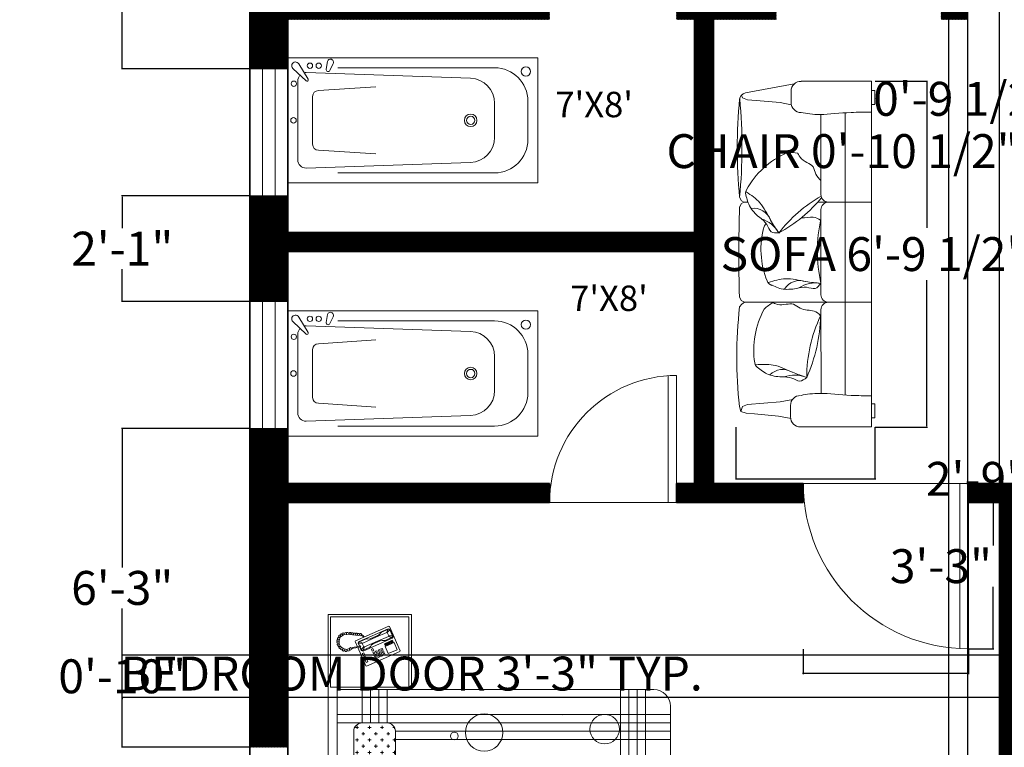
# Model space of a CAD drawing. Units: inches. Extents: x 108 to 771, y 58 to 590.
# Tile 2 of 8: x 108 to 341, y 231 to 402. Entities that reach past the tile are written whole.
import ezdxf

# ---------------------------------------------------------------- set-up
doc = ezdxf.new("R2010")
doc.units = ezdxf.units.IN
doc.header["$MEASUREMENT"] = 0
for name, color, linetype, lineweight in [('A-ANNO-DIMS', 2, 'Continuous', 13), ('A-AREA-IDEN', 7, 'Continuous', 18), ('A-DOOR', 3, 'Continuous', 18), ('A-FLOR-FIXT', 8, 'Continuous', 15), ('A-GLAZ', 4, 'Continuous', 18), ('A-WALL', 7, 'Continuous', 35), ('A-WALL-PATT', 252, 'Continuous', 9), ('Furniture', 7, 'Continuous', 15)]:
    doc.layers.add(name, color=color, linetype=linetype, lineweight=lineweight)
doc.styles.get("Standard").update_dxf_attribs({"font": 'italic8.shx'})
doc.dimstyles.get("Standard").update_dxf_attribs({"dimtxt": 8, "dimasz": 0.18, "dimexe": 0.18, "dimexo": 0.0625, "dimgap": 0.09, "dimtad": 0, "dimtih": 1, "dimtoh": 1, "dimzin": 0, "dimdsep": 46, "dimlunit": 3, "dimtxsty": 'Standard', "dimcen": 0.09, "dimclrt": 6, "dimadec": 0, "dimazin": 0, "dimtfac": 1, "dimtofl": 0, "dimtmove": 0, "dimatfit": 3, "dimfxl": 1, "dimtolj": 1, "dimtzin": 0, "dimarcsym": 0})

# ---------------------------------------------------------------- blocks, each defined once
blk = doc.blocks.new('DOOR-SINGLE-39')
for p, q in [((0, 39), (0, 0)), ((2, 38.95), (2, 0)), ((0, 0), (39, 0))]:
    blk.add_line(p, q)
blk.add_arc((0, 0), 39, 0, 90)
blk = doc.blocks.new('DOOR-SINGLE-30')
for p, q in [((28, 29.93), (28, 0)), ((30, 30), (30, 0)), ((30, 0), (0, 0))]:
    blk.add_line(p, q)
blk.add_arc((30, 0), 30, 90, 180)
blk = doc.blocks.new('WINDOW-30')
for p, q in [((0, 0), (0, 30)), ((0, 30), (9, 30)), ((3, 30), (3, 0)), ((6, 30), (6, 0)), ((9, 30), (9, 0)), ((9, 0), (0, 0))]:
    blk.add_line(p, q)
blk = doc.blocks.new('BED-WITH-NIGHTSTANDS')
h = blk.add_hatch()
h.set_pattern_fill('CROSS', color=256, scale=5.9055, angle=450, style=0)
h.set_pattern_definition([(90, (-724.7189, -618.2251), (1.476375, 1.476375), [0.7381875, -2.2145625]), (360, (-725.088, -617.856), (1.476375, -1.476375), [0.7381875, -2.2145625])])
h.paths.add_polyline_path([(13.93, 48.57), (8.02, 48.57, 0.414214), (6.06, 46.6), (6.06, 28.74, 0.414214), (8.02, 26.77), (13.93, 26.77, 0.414214), (15.9, 28.74), (15.9, 46.6, 0.414214)])
h.paths.add_polyline_path([(6.06, 62.99, 0.19223), (8.02, 57.33), (13.93, 57.33, 0.19223), (15.9, 62.99), (15.9, 78.74, 0.414214), (13.93, 80.71), (8.02, 80.71, 0.414214), (6.06, 78.74)])
for p, q in [((0, 0), (0, 106.3)), ((19.69, 106.3), (0, 106.3)), ((19.09, 105.71), (0.59, 105.71)), ((0.59, 105.71), (0.59, 89.17)), ((19.09, 105.71), (19.09, 89.17)), ((19.69, 106.3), (19.69, 88.58)), ((14.35, 103.55), (6.45, 100.09)), ((14.21, 102.94), (7.34, 99.94)), ((14.14, 102.78), (12.6, 102.1)), ((14.14, 102.78), (13.85, 102.03)), ((13.99, 102.03), (14.61, 102.64)), ((14.4, 102.82), (14.14, 102.78)), ((14.62, 102.78), (14.21, 102.94)), ((14.52, 103.48), (14.35, 103.55)), ((14.61, 102.64), (14.4, 102.82)), ((17.02, 97.76), (14.52, 103.48)), ((15.21, 101.26), (14.61, 102.64)), ((15.37, 101.06), (14.62, 102.78)), ((2.06, 100.15), (2.14, 100.41)), ((2.46, 100.04), (2.06, 100.15)), ((2.1, 99.92), (2.46, 100.04)), ((2.14, 100.41), (2.51, 100.41)), ((2.23, 100.67), (2.3, 100.88)), ((2.51, 100.41), (2.23, 100.67)), ((2.3, 100.88), (2.69, 100.86)), ((2.44, 101.15), (2.63, 101.34)), ((2.69, 100.86), (2.44, 101.15)), ((2.89, 100.92), (2.62, 100.19)), ((2.62, 100.19), (2.62, 99.39)), ((2.63, 101.34), (3.06, 101.2)), ((2.89, 101.55), (3.11, 101.7)), ((3.06, 101.2), (2.89, 101.55)), ((3.69, 101.46), (2.89, 100.92)), ((3.11, 101.7), (3.41, 101.48)), ((3.36, 101.88), (3.67, 101.95)), ((3.41, 101.48), (3.36, 101.88)), ((3.67, 101.95), (3.81, 101.64)), ((4.95, 101.56), (3.69, 101.46)), ((3.81, 101.64), (3.94, 101.98)), ((3.94, 101.98), (4.24, 102.02)), ((4.24, 102.02), (4.39, 101.64)), ((4.37, 102.03), (4.76, 102.08)), ((4.39, 101.64), (4.37, 102.03)), ((4.76, 102.08), (4.88, 101.72)), ((4.88, 101.72), (5.13, 102.07)), ((5.79, 101.48), (4.95, 101.56)), ((5.13, 102.07), (5.37, 102.03)), ((5.37, 102.03), (5.42, 101.66)), ((5.42, 101.66), (5.65, 101.97)), ((5.65, 101.97), (5.95, 101.95)), ((5.86, 101.55), (5.79, 101.48)), ((5.92, 101.48), (5.86, 101.55)), ((6.5, 101.45), (5.92, 101.48)), ((5.95, 101.95), (5.98, 101.59)), ((5.98, 101.59), (6.16, 101.92)), ((6.16, 101.92), (6.47, 101.91)), ((6.45, 100.09), (6.38, 99.93)), ((6.47, 101.91), (6.46, 101.54)), ((6.46, 101.54), (6.62, 101.9)), ((7.29, 101.35), (6.5, 101.45)), ((6.62, 101.9), (6.85, 101.89)), ((6.85, 101.89), (6.89, 101.51)), ((6.89, 101.51), (7.15, 101.84)), ((7.15, 101.84), (7.36, 101.82)), ((7.73, 101.29), (7.29, 101.35)), ((7.36, 101.82), (7.4, 101.48)), ((7.4, 101.48), (7.62, 101.8)), ((7.44, 99.85), (8.99, 100.52)), ((7.62, 101.8), (7.77, 101.81)), ((7.79, 101.48), (7.73, 101.29)), ((7.77, 101.81), (7.86, 101.7)), ((7.84, 101.37), (7.79, 101.48)), ((7.94, 101.33), (7.84, 101.37)), ((7.86, 101.7), (7.96, 101.49)), ((8.11, 101.22), (7.94, 101.33)), ((7.96, 101.49), (8.25, 101.43)), ((8.26, 101.14), (8.11, 101.22)), ((11.28, 100.91), (8.18, 99.56)), ((8.25, 101.43), (8.4, 101.32)), ((8.4, 100.95), (8.26, 101.14)), ((8.26, 97.68), (15.18, 100.71)), ((8.4, 101.32), (8.57, 101.02)), ((11.68, 99.99), (8.58, 98.64)), ((8.99, 100.52), (9.33, 100.53)), ((9.33, 100.53), (9.69, 100.49)), ((9.69, 100.49), (10.11, 100.6)), ((10.11, 100.6), (11.2, 101.08)), ((11.77, 101.33), (11.2, 101.08)), ((11.28, 100.91), (13.85, 102.03)), ((11.68, 99.99), (14.25, 101.12)), ((12.33, 100.07), (11.75, 99.82)), ((12.15, 101.56), (11.77, 101.33)), ((12.36, 101.86), (12.15, 101.56)), ((12.75, 100.19), (12.33, 100.07)), ((12.6, 102.1), (12.36, 101.86)), ((13.11, 100.14), (12.75, 100.19)), ((13.45, 100.15), (13.11, 100.14)), ((15, 100.83), (13.45, 100.15)), ((13.85, 102.03), (13.99, 102.03)), ((13.99, 102.03), (14.34, 101.23)), ((14.25, 101.12), (14.34, 101.23)), ((15, 100.83), (14.25, 101.12)), ((14.34, 101.23), (15.21, 101.26)), ((14.67, 100), (14.84, 100.08)), ((14.87, 99.55), (14.67, 100)), ((14.84, 100.08), (15.04, 99.62)), ((15.2, 100.99), (15, 100.83)), ((15.02, 100.16), (15.19, 100.23)), ((15.22, 99.7), (15.02, 100.16)), ((15.18, 100.71), (15.37, 101.06)), ((15.19, 100.23), (15.39, 99.77)), ((15.21, 101.26), (15.2, 100.99)), ((2.09, 99.7), (2.1, 99.92)), ((2.44, 99.53), (2.09, 99.7)), ((2.13, 99.38), (2.44, 99.53)), ((2.17, 99.14), (2.13, 99.38)), ((2.59, 99.17), (2.17, 99.14)), ((2.29, 98.95), (2.59, 99.17)), ((2.4, 98.76), (2.29, 98.95)), ((2.78, 98.76), (2.4, 98.76)), ((2.53, 98.47), (2.78, 98.76)), ((2.71, 98.26), (2.53, 98.47)), ((2.62, 99.39), (2.98, 98.72)), ((3.07, 98.46), (2.71, 98.26)), ((2.96, 98.08), (3.07, 98.46)), ((3.2, 97.92), (2.96, 98.08)), ((2.98, 98.72), (3.58, 98.25)), ((3.49, 98.1), (3.2, 97.92)), ((3.41, 97.75), (3.49, 98.1)), ((3.69, 97.67), (3.41, 97.75)), ((3.58, 98.25), (4.33, 98.05)), ((3.95, 97.97), (3.69, 97.67)), ((4.03, 97.59), (3.95, 97.97)), ((4.33, 98.05), (5.08, 98.31)), ((4.48, 97.99), (4.36, 97.56)), ((4.67, 97.64), (4.48, 97.99)), ((5, 97.75), (4.67, 97.64)), ((5.05, 98.16), (5, 97.75)), ((5.26, 97.85), (5.05, 98.16)), ((5.08, 98.31), (5.33, 98.48)), ((5.53, 98), (5.26, 97.85)), ((5.33, 98.48), (5.57, 98.34)), ((5.6, 98.18), (5.53, 98)), ((5.57, 98.34), (5.87, 98.48)), ((5.68, 98.18), (5.6, 98.18)), ((5.98, 98.32), (5.68, 98.18)), ((5.87, 98.48), (6.16, 98.57)), ((6.58, 98.42), (5.98, 98.32)), ((6.16, 98.57), (6.77, 98.66)), ((6.38, 99.93), (6.92, 98.7)), ((7.22, 98.53), (6.58, 98.42)), ((6.77, 98.66), (7.17, 98.75)), ((7.01, 98.5), (8.89, 94.2)), ((7.34, 99.94), (7.12, 99.5)), ((7.12, 99.5), (7.41, 98.83)), ((7.17, 98.75), (7.65, 98.91)), ((7.72, 98.74), (7.22, 98.53)), ((7.23, 99.41), (7.24, 99.69)), ((8.09, 99.45), (7.23, 99.41)), ((7.47, 98.85), (7.23, 99.41)), ((7.24, 99.69), (7.44, 99.85)), ((7.44, 99.85), (8.18, 99.56)), ((7.49, 98.64), (7.84, 97.84)), ((7.83, 98.04), (7.55, 98.67)), ((7.65, 98.91), (7.72, 98.74)), ((8.45, 98.65), (7.83, 98.04)), ((7.83, 98.04), (8.04, 97.86)), ((7.84, 97.84), (8.26, 97.68)), ((8.04, 97.86), (8.29, 97.9)), ((8.18, 99.56), (8.09, 99.45)), ((8.09, 99.45), (8.45, 98.65)), ((8.29, 97.9), (8.58, 98.64)), ((8.29, 97.9), (9.84, 98.58)), ((8.58, 98.64), (8.45, 98.65)), ((9.84, 98.58), (10.08, 98.82)), ((10.08, 98.82), (10.29, 99.11)), ((10.58, 98.29), (10.24, 98.14)), ((10.24, 98.14), (10.44, 97.68)), ((10.29, 99.11), (10.66, 99.34)), ((10.44, 97.68), (10.78, 97.83)), ((10.78, 97.83), (10.58, 98.29)), ((10.66, 99.34), (11.75, 99.82)), ((11.56, 97.76), (11.22, 97.61)), ((11.71, 97.42), (11.56, 97.76)), ((12.19, 98.03), (11.85, 97.88)), ((11.85, 97.88), (12, 97.54)), ((12, 97.54), (12.34, 97.69)), ((12.34, 97.69), (12.19, 98.03)), ((12.82, 98.31), (12.48, 98.16)), ((12.48, 98.16), (12.63, 97.82)), ((12.63, 97.82), (12.97, 97.97)), ((13.07, 97.74), (12.73, 97.59)), ((12.97, 97.97), (12.82, 98.31)), ((13.22, 97.39), (13.07, 97.74)), ((13.3, 99.4), (13.47, 99.48)), ((13.5, 98.95), (13.3, 99.4)), ((15.58, 99.65), (13.46, 98.72)), ((13.46, 98.72), (14.18, 97.06)), ((13.47, 99.48), (13.67, 99.02)), ((13.67, 99.02), (13.5, 98.95)), ((13.64, 99.55), (13.81, 99.63)), ((13.84, 99.1), (13.64, 99.55)), ((13.81, 99.63), (14.01, 99.17)), ((14.01, 99.17), (13.84, 99.1)), ((13.99, 99.7), (14.16, 99.78)), ((14.19, 99.25), (13.99, 99.7)), ((14.16, 99.78), (14.36, 99.32)), ((14.18, 97.06), (16.3, 97.99)), ((14.36, 99.32), (14.19, 99.25)), ((14.33, 99.85), (14.5, 99.93)), ((14.53, 99.4), (14.33, 99.85)), ((14.5, 99.93), (14.7, 99.47)), ((14.7, 99.47), (14.53, 99.4)), ((15.04, 99.62), (14.87, 99.55)), ((15.39, 99.77), (15.22, 99.7)), ((16.3, 97.99), (15.58, 99.65)), ((16.96, 97.59), (17.02, 97.76)), ((4.36, 97.56), (4.03, 97.59)), ((8.09, 97.13), (8.43, 97.28)), ((8.34, 96.55), (8.09, 97.13)), ((8.68, 96.7), (8.34, 96.55)), ((8.43, 97.28), (8.68, 96.7)), ((8.44, 96.33), (8.78, 96.48)), ((8.69, 95.75), (8.44, 96.33)), ((9.03, 95.9), (8.69, 95.75)), ((8.78, 96.48), (9.03, 95.9)), ((8.79, 95.52), (9.13, 95.67)), ((9.04, 94.95), (8.79, 95.52)), ((9.05, 94.14), (16.96, 97.59)), ((9.13, 95.67), (9.38, 95.1)), ((10.93, 97.48), (10.59, 97.33)), ((10.59, 97.33), (10.74, 96.99)), ((10.74, 96.99), (11.08, 97.14)), ((11.18, 96.91), (10.84, 96.76)), ((10.84, 96.76), (10.99, 96.42)), ((11.08, 97.14), (10.93, 97.48)), ((10.99, 96.42), (11.33, 96.57)), ((11.43, 96.34), (11.09, 96.19)), ((11.09, 96.19), (11.24, 95.84)), ((11.33, 96.57), (11.18, 96.91)), ((11.22, 97.61), (11.37, 97.27)), ((11.24, 95.84), (11.58, 95.99)), ((11.37, 97.27), (11.71, 97.42)), ((11.58, 95.99), (11.43, 96.34)), ((11.81, 97.19), (11.47, 97.04)), ((11.47, 97.04), (11.62, 96.69)), ((11.62, 96.69), (11.96, 96.84)), ((12.06, 96.61), (11.72, 96.46)), ((11.72, 96.46), (11.87, 96.12)), ((11.96, 96.84), (11.81, 97.19)), ((11.87, 96.12), (12.21, 96.27)), ((12.21, 96.27), (12.06, 96.61)), ((12.44, 97.46), (12.1, 97.31)), ((12.1, 97.31), (12.25, 96.97)), ((12.25, 96.97), (12.59, 97.12)), ((12.69, 96.89), (12.35, 96.74)), ((12.35, 96.74), (12.5, 96.39)), ((12.59, 97.12), (12.44, 97.46)), ((12.5, 96.39), (12.84, 96.55)), ((12.84, 96.55), (12.69, 96.89)), ((12.73, 97.59), (12.88, 97.24)), ((12.88, 97.24), (13.22, 97.39)), ((13.32, 97.16), (12.98, 97.01)), ((12.98, 97.01), (13.13, 96.67)), ((13.13, 96.67), (13.47, 96.82)), ((13.47, 96.82), (13.32, 97.16)), ((8.89, 94.2), (9.05, 94.14)), ((9.38, 95.1), (9.04, 94.95)), ((19.09, 89.17), (0.59, 89.17)), ((0.59, 89.17), (19.09, 89.17)), ((2.12, 17.72), (2.12, 88.58)), ((2.12, 88.58), (76.92, 88.58)), ((80.86, 84.65), (80.86, 21.65)), ((55.34, 82.68), (55.28, 82.62)), ((6.07, 78.98), (6.07, 62.76)), ((6.07, 46.84), (6.07, 28.51)), ((6.07, 44.57), (6.06, 44.56)), ((50.36, 26.51), (46.1, 22.26)), ((19.09, 17.13), (0.59, 17.13)), ((0.59, 0.59), (0.59, 17.13)), ((76.92, 17.72), (2.12, 17.72)), ((19.09, 0.59), (19.09, 17.13)), ((19.69, 0), (19.69, 17.72)), ((9.61, 8.71), (9.61, 14.05)), ((8.07, 10.1), (5.65, 12.3)), ((11, 10.24), (13.2, 12.67)), ((9.61, 8.71), (4.26, 8.71)), ((8.22, 7.18), (6.02, 4.75)), ((9.61, 8.71), (14.95, 8.71)), ((9.61, 8.71), (9.61, 3.36)), ((11.14, 7.32), (13.56, 5.12)), ((19.69, 0), (0, 0)), ((19.09, 0.59), (0.59, 0.59))]:
    blk.add_line(p, q)
for points in [[(8.02, 88.58), (8.02, 80.71)], [(9.99, 80.71), (9.99, 88.58), (8.02, 88.58)], [(13.93, 80.71), (13.93, 88.58), (11.96, 88.58)], [(11.96, 88.58), (11.96, 80.71)], [(2.12, 80.71), (80.86, 80.71), (80.86, 82.68), (2.12, 82.68)], [(15.9, 76.77), (80.86, 76.77), (80.86, 78.74), (15.9, 78.74)], [(8.02, 57.33), (8.02, 48.57)], [(9.99, 48.57), (9.99, 57.33)], [(11.96, 57.33), (11.96, 48.57)], [(13.93, 48.57), (13.93, 57.33)], [(2.12, 29.53), (6.06, 29.53)], [(15.9, 29.53), (80.86, 29.53), (80.86, 27.56), (15.9, 27.56)], [(6.06, 27.56), (2.12, 27.56)], [(2.12, 25.59), (80.86, 25.59), (80.86, 23.62), (2.12, 23.62)], [(8.02, 25.59), (8.02, 17.72), (9.99, 17.72), (9.99, 25.59)], [(11.96, 25.59), (11.96, 17.72), (13.93, 17.72), (13.93, 25.59)]]:
    blk.add_lwpolyline(points)
for points in [[(69.05, 88.58), (69.05, 17.72), (71.02, 17.72), (71.02, 88.58)], [(72.98, 88.58), (72.98, 17.72), (74.95, 17.72), (74.95, 88.58)]]:
    blk.add_lwpolyline(points, close=True)
for points in [[(15.9, 62.99), (15.9, 78.74, 0.414214), (13.93, 80.71), (8.02, 80.71, 0.414214), (6.06, 78.74), (6.06, 62.99, 0.19223), (8.02, 57.33), (13.93, 57.33, 0.19223)], [(15.9, 28.74), (15.9, 46.6, 0.414214), (13.93, 48.57), (8.02, 48.57, 0.414214), (6.06, 46.6), (6.06, 28.74, 0.414214), (8.02, 26.77), (13.93, 26.77, 0.414214)]]:
    blk.add_lwpolyline(points, format="xyb", close=True)
for centre, radius in [((36.86, 78.44), 4.41), ((65.32, 79.25), 3.48), ((29.81, 77.62), 0.925), ((20.97, 68.13), 2.09), ((65.3, 65.16), 2.09), ((68.02, 44.43), 4.65), ((28.31, 37.66), 4.65), ((46.05, 37.48), 0.925), ((60.91, 32.6), 1.14), ((71.58, 30.51), 2.09), ((46.4, 25.43), 3.19), ((9.61, 8.71), 5.54), ((9.61, 8.71), 5.34), ((9.61, 8.71), 2.07)]:
    blk.add_circle(centre, radius)
for centre, start, end in [((76.92, 84.65), 0, 90), ((76.92, 21.65), 270, 0)]:
    blk.add_arc(centre, 3.94, start, end)
blk = doc.blocks.new('BATHTUB')
for p, q in [((59.06, 29.53), (0, 29.53)), ((0, 29.53), (0, 0)), ((4.78, 24.45), (2.59, 28.08)), ((9.35, 28.65), (9.04, 26.82)), ((9.94, 26.54), (10.7, 28.16)), ((59.06, 0), (59.06, 29.53)), ((1.15, 27.02), (4.3, 24.06)), ((4.33, 26.04), (43.12, 24.68)), ((48.82, 27.17), (11.81, 27.17)), ((2.36, 24.07), (2.36, 5.46)), ((7.23, 21.79), (20.76, 22.69)), ((5.85, 20.41), (5.85, 9.11)), ((48.82, 10.75), (48.82, 19.29)), ((56.69, 10.24), (56.69, 19.29)), ((7.23, 7.74), (20.76, 6.84)), ((4.33, 3.49), (43.12, 4.85)), ((11.81, 2.36), (48.82, 2.36)), ((0, 0), (59.06, 0))]:
    blk.add_line(p, q)
for centre, radius in [((5.23, 27.66), 0.628), ((7.29, 27.66), 0.628), ((56.21, 26.29), 1.09), ((1.42, 23.41), 0.628), ((1.34, 14.76), 0.656), ((43.18, 14.76), 1.48), ((43.18, 14.76), 0.984)]:
    blk.add_circle(centre, radius)
for centre, radius, start, end in [((1.81, 27.63), 0.903, 29.9808, 223.0225), ((10.05, 28.48), 0.722, 333.7022, 166.7439), ((4.33, 24.07), 1.97, 90, 103.842), ((4.33, 24.07), 1.97, 90, 103.842), ((9.51, 26.74), 0.472, 170.4963, 334.8002), ((48.82, 19.29), 7.87, 0, 90), ((4.33, 24.07), 1.97, 137.6863, 180), ((4.33, 24.07), 1.97, 137.6863, 180), ((4.51, 24.29), 0.315, 226.7749, 31.0788), ((4.51, 24.29), 0.315, 226.7749, 31.0788), ((42.91, 18.78), 5.91, 0, 87.9984), ((7.23, 20.41), 1.38, 90, 180), ((42.91, 10.75), 5.91, 272.0016, 0), ((48.82, 10.24), 7.87, 270, 0), ((7.23, 9.11), 1.38, 180, 270), ((4.33, 5.46), 1.97, 180, 270)]:
    blk.add_arc(centre, radius, start, end)
blk = doc.blocks.new('SOFA')
for p, q in [((31.83, 81.57, 13.5), (15.2, 81.57, 13.5)), ((31.83, 81.57, 13.5), (31.83, 0)), ((13.53, 80.95), (2.06, 78.82)), ((12.83, 79.28), (12.82, 76.57)), ((31.83, 79.37, 0.36), (32.62, 79.37, 0.36)), ((32.62, 79.37, 0.36), (32.62, 76.1, 0.36)), ((1.33, 77.65), (1.12, 78.32)), ((2.53, 77.19), (1.33, 77.65)), ((4.58, 77.03), (2.53, 77.19)), ((10.24, 76.55), (4.58, 77.03)), ((12.88, 76.04), (10.24, 76.55)), ((32.62, 76.1, 0.36), (31.83, 76.1, 0.91)), ((19.88, 73.73), (19.88, 54.83)), ((25.57, 7.53, 9.89), (25.57, 74.14, 9.89)), ((1.09, 53.34), (0.67, 54.21)), ((1.09, 52.77), (0.68, 51.91)), ((1.64, 53.06), (1.09, 53.34)), ((1.64, 53.06), (1.09, 52.77)), ((1.64, 53.06), (2.64, 53.06)), ((19.09, 53.06), (21.65, 53.06)), ((19.88, 51.29), (19.88, 31.21)), ((21.65, 53.06), (31.83, 53.06)), ((1.05, 29.87), (0.64, 30.74)), ((1.19, 29.01), (0.68, 28.32)), ((1.8, 29.44), (1.05, 29.87)), ((1.81, 29.44), (1.19, 29.01)), ((26.18, 29.43), (1.8, 29.43)), ((31.83, 29.43), (21.65, 29.43)), ((19.88, 27.66), (19.89, 7.88, 0.34)), ((0.97, 3.69), (0.62, 4.84)), ((1.33, 4.84), (0.97, 3.69)), ((2.53, 5.3), (1.33, 4.84)), ((10.24, 5.94), (2.53, 5.3)), ((13.2, 6.51), (10.24, 5.94)), ((12.69, 2.37), (12.69, 5.08)), ((32.62, 5.47, 0.36), (31.83, 5.47, 0.91)), ((32.62, 2.2, 0.36), (32.62, 5.47, 0.36)), ((2.18, 3.23), (0.97, 3.69)), ((4.22, 3.07), (2.18, 3.23)), ((9.88, 2.59), (4.22, 3.07)), ((12.84, 2.01), (9.88, 2.59)), ((15.05, 0.01), (31.83, 0)), ((31.83, 2.2, 0.36), (32.62, 2.2, 0.36))]:
    blk.add_line(p, q)
for centre, radius, start, end in [((15.09, 79.31, 13.5), 2.25, 87.0581, 180.9206), ((123.26, 65.95), 123.14, 174.6632, 185.4698), ((2.39, 77.08), 1.77, 100.5091, 180), ((-121.91, 65.95), 123.14, 354.5302, 5.3368), ((15.19, 76.56), 2.36, 179.7859, 269.7859), ((19.84, 46.39, 13.5), 19.99, 113.7986, 151.3924), ((12.86, 58.3, 13.5), 6.47, 76.1804, 99.6612), ((3.85, 55.11, 13.5), 1.77, 151.3924, 203.2188), ((36.72, 25.19, 13.5), 33.78, 119.8342, 142.4564), ((-6.19, 75.47, 13.5), 33.78, 298.4934, 321.1155), ((21.65, 54.83), 1.77, 180, 270), ((315.61, 40.74), 315.13, 177.9678, 181.8181), ((3.98, 47.34, 13.5), 4.27, 21.4614, 98.0497), ((21.65, 51.29), 1.77, 90, 180), ((3.65, 42.24, 13.5), 7.21, 29.4203, 72.7126), ((52.79, 41.52, 13.5), 33.78, 166.9593, 193.0407), ((25.7, 41.94, 13.5), 19.99, 164.3829, 201.9767), ((12.07, 44.11, 13.5), 6.47, 142.7695, 150.2454), ((8.8, 35.12, 13.5), 1.77, 201.9767, 253.8031), ((14.9, 30.29, 13.5), 4.27, 72.0456, 148.634), ((18.62, 26.79, 13.5), 7.21, 80.0046, 123.2969), ((21.65, 31.21), 1.77, 180, 270), ((107.05, 16.32), 107.05, 173.5605, 186.1533), ((11.21, 23.4, 13.5), 6.47, 113.6986, 137.1794), ((21.65, 27.66), 1.77, 90, 180), ((24, 18.21, 13.5), 19.99, 151.3169, 188.9106), ((-18.44, 27.22, 13.5), 38.25, 336.0331, 358.4688), ((50.29, 11.67, 13.5), 33.78, 154.5272, 179.9746), ((6, 15.39, 13.5), 1.77, 188.9106, 240.7371), ((10.84, 9.3, 13.5), 4.27, 58.9796, 135.568), ((13.68, 5.05, 13.5), 7.21, 66.9386, 110.2309), ((15.05, 5.08), 2.36, 90, 180), ((15.05, 2.37), 2.36, 180, 269.9816)]:
    blk.add_arc(centre, radius, start, end)
for points, knots in [([(15.18, 74.2), (16.54, 73.96, 2.2), (19.42, 73.44, 6.84), (25.93, 74.31, 10.25), (30.21, 74.29, 11.73), (31.83, 74.28, 12.29)], [0, 0, 0, 0, 7.670782, 16.13452, 21.306634, 21.306634, 21.306634, 21.306634]), ([(14.41, 64.59, 13.5), (14.41, 64.59, 13.5), (15.3, 62.57, 13.5), (18.13, 62.25, 13.5), (18.49, 59.48, 13.5), (19.41, 58.61, 13.5), (19.88, 58.17, 13.5)], [27.786417, 27.786417, 27.786417, 27.786417, 60.334214, 153.42843, 198.910048, 250.027656, 250.027656, 250.027656, 250.027656]), ([(2.08, 55.2, 13.5), (2.3, 54.16, 13.5), (2.79, 51.93, 13.5), (4.99, 49.65, 13.5), (7.18, 48.12, 13.5), (7.83, 45.76, 13.5), (9.25, 45.77, 13.5), (9.93, 45.78, 13.5)], [0, 0, 0, 0, 3.139621, 6.721226, 9.134784, 11.147372, 12.969489, 12.969489, 12.969489, 12.969489]), ([(2.23, 55.48, 13.5), (3.39, 54.7, 13.5), (5.91, 53.01, 13.5), (7.71, 49.11, 13.5), (9.26, 46.77, 13.5), (9.93, 45.78, 13.5)], [0, 0, 0, 0, 4.104513, 8.93575, 12.539242, 12.539242, 12.539242, 12.539242]), ([(15.26, 49.37, 13.5), (16.21, 49.3, 13.5), (17.85, 49.84, 13.5), (19.2, 49.22, 13.5), (19.79, 48.78, 13.5)], [214.332348, 214.332348, 214.332348, 214.332348, 289.238615, 341.466319, 341.466319, 341.466319, 341.466319]), ([(7.49, 34.11, 13.5), (8.83, 34.51, 13.5), (11.73, 35.38, 13.5), (15.9, 34.29, 13.5), (18.69, 34.01, 13.5), (19.88, 33.9, 13.5)], [0, 0, 0, 0, 4.104513, 8.93575, 12.539242, 12.539242, 12.539242, 12.539242]), ([(7.62, 33.81, 13.5), (8.56, 33.33, 13.5), (10.59, 32.29, 13.5), (13.75, 32.54, 13.5), (16.32, 33.26, 13.5), (18.56, 32.26, 13.5), (19.45, 33.37, 13.5), (19.88, 33.9, 13.5)], [0, 0, 0, 0, 3.139621, 6.721226, 9.134784, 11.147372, 12.969489, 12.969489, 12.969489, 12.969489]), ([(8.61, 29.33, 13.5), (8.61, 29.33, 13.5), (10.55, 28.27, 13.5), (12.98, 29.74, 13.5), (15.37, 27.37, 13.5), (18, 27.79, 13.5), (19.32, 26.76, 13.5), (19.79, 26.2, 13.5)], [27.786417, 27.786417, 27.786417, 27.786417, 60.334214, 153.42843, 198.910048, 289.238615, 341.466319, 341.466319, 341.466319, 341.466319]), ([(4.5, 14.7, 13.5), (5.89, 14.78, 13.5), (8.91, 14.98, 13.5), (12.72, 12.97, 13.5), (15.38, 12.07, 13.5), (16.51, 11.69, 13.5)], [0, 0, 0, 0, 4.104513, 8.93575, 12.539242, 12.539242, 12.539242, 12.539242]), ([(4.55, 14.37, 13.5), (5.36, 13.69, 13.5), (7.1, 12.22, 13.5), (10.24, 11.75, 13.5), (12.91, 11.87, 13.5), (14.86, 10.39, 13.5), (15.98, 11.27, 13.5), (16.51, 11.69, 13.5)], [0, 0, 0, 0, 3.139621, 6.721226, 9.134784, 11.147372, 12.969489, 12.969489, 12.969489, 12.969489]), ([(15.18, 7.47), (16.54, 7.71, 2.2), (19.42, 8.23, 6.84), (25.93, 7.36, 10.25), (30.21, 7.38, 11.73), (31.83, 7.39, 12.29)], [0, 0, 0, 0, 7.670782, 16.13452, 21.306634, 21.306634, 21.306634, 21.306634])]:
    blk.add_open_spline(points, degree=3, knots=knots)
blk = doc.blocks.new('*D28')
at = {"layer": 'A-ANNO-DIMS', "color": 0, "lineweight": -2, "transparency": 16777216}
for p, q in [((293.04, 253.99), (293.04, 248.02)), ((332.04, 253.99), (332.04, 248.02)), ((293.04, 248.2), (292.86, 248.2)), ((331.86, 248.2), (293.22, 248.2))]:
    blk.add_line(p, q, dxfattribs=at)
at = {"layer": 'A-ANNO-DIMS', "color": 0, "transparency": 16777216}
for points in [[(293.22, 248.23), (293.22, 248.17), (293.04, 248.2)], [(331.86, 248.23), (331.86, 248.17), (332.04, 248.2)]]:
    blk.add_solid(points, dxfattribs=at)
at = {"layer": 'Defpoints', "color": 0, "transparency": 16777216}
for p in [(293.04, 254.05), (332.04, 254.05), (293.04, 248.2)]:
    blk.add_point(p, dxfattribs=at)
at = {"layer": 'A-ANNO-DIMS', "color": 6, "transparency": 16777216, "insert": (200.58, 248.2), "char_height": 8, "attachment_point": 5}
blk.add_mtext('\\A1;BEDROOM DOOR 3\'-3" TYP.', dxfattribs=at)
blk = doc.blocks.new('*D29')
at = {"layer": 'A-ANNO-DIMS', "color": 0, "lineweight": -2, "transparency": 16777216}
for p, q in [((332.1, 293.05), (338.07, 293.05)), ((337.89, 292.87), (337.89, 278.4)), ((337.89, 254.23), (337.89, 268.7)), ((332.1, 254.05), (338.07, 254.05))]:
    blk.add_line(p, q, dxfattribs=at)
at = {"layer": 'A-ANNO-DIMS', "color": 0, "transparency": 16777216}
for points in [[(337.86, 292.87), (337.92, 292.87), (337.89, 293.05)], [(337.86, 254.23), (337.92, 254.23), (337.89, 254.05)]]:
    blk.add_solid(points, dxfattribs=at)
at = {"layer": 'Defpoints', "color": 0, "transparency": 16777216}
for p in [(332.04, 293.05), (332.04, 254.05), (337.89, 254.05)]:
    blk.add_point(p, dxfattribs=at)
at = {"layer": 'A-ANNO-DIMS', "color": 6, "transparency": 16777216, "insert": (337.89, 273.55), "char_height": 8, "attachment_point": 5}
blk.add_mtext('\\A1;3\'-3" TYP.', dxfattribs=at)
blk = doc.blocks.new('*D32')
at = {"layer": 'A-ANNO-DIMS', "color": 0, "lineweight": -2, "transparency": 16777216}
for p, q in [((395.01, 382.23), (393.3, 382.24)), ((393.48, 382.06), (393.42, 371.84)), ((394.94, 371.65), (393.24, 371.66)), ((393.42, 371.48), (393.24, 371.48)), ((393.42, 371.66), (393.42, 371.48))]:
    blk.add_line(p, q, dxfattribs=at)
at = {"layer": 'A-ANNO-DIMS', "color": 0, "transparency": 16777216}
for points in [[(393.45, 382.06), (393.51, 382.06), (393.48, 382.24)], [(393.39, 371.84), (393.45, 371.84), (393.42, 371.66)]]:
    blk.add_solid(points, dxfattribs=at)
at = {"layer": 'Defpoints', "color": 0, "transparency": 16777216}
for p in [(395.07, 382.23), (393.42, 371.66), (395.01, 371.65)]:
    blk.add_point(p, dxfattribs=at)
at = {"layer": 'A-ANNO-DIMS', "color": 6, "transparency": 16777216, "insert": (314.67, 371.48), "char_height": 8, "attachment_point": 5}
blk.add_mtext('\\A1;CHAIR 0\'-10 1/2" TYP.', dxfattribs=at)
blk = doc.blocks.new('*D33')
at = {"layer": 'A-ANNO-DIMS', "color": 0, "lineweight": -2, "transparency": 16777216}
for p, q in [((395.08, 383.82), (394.9, 383.82)), ((395.07, 382.3), (395.08, 384)), ((404.44, 383.77), (395.26, 383.82)), ((404.61, 382.24), (404.62, 383.94))]:
    blk.add_line(p, q, dxfattribs=at)
at = {"layer": 'A-ANNO-DIMS', "color": 0, "transparency": 16777216}
for points in [[(395.26, 383.85), (395.26, 383.79), (395.08, 383.82)], [(404.44, 383.8), (404.44, 383.74), (404.62, 383.76)]]:
    blk.add_solid(points, dxfattribs=at)
at = {"layer": 'Defpoints', "color": 0, "transparency": 16777216}
for p in [(395.08, 383.82), (395.07, 382.23), (404.61, 382.18)]:
    blk.add_point(p, dxfattribs=at)
at = {"layer": 'A-ANNO-DIMS', "color": 6, "transparency": 16777216, "insert": (343.38, 383.82), "char_height": 8, "attachment_point": 5}
blk.add_mtext('\\A1;0\'-9 1/2" TYP.', dxfattribs=at)
blk = doc.blocks.new('*D44')
at = {"layer": 'A-ANNO-DIMS', "color": 0, "lineweight": -2, "transparency": 16777216}
for p, q in [((310.02, 387.98), (322.38, 387.98)), ((322.2, 387.8), (322.2, 353.37)), ((322.2, 306.56), (322.2, 341)), ((310.02, 306.38), (322.38, 306.38))]:
    blk.add_line(p, q, dxfattribs=at)
at = {"layer": 'A-ANNO-DIMS', "color": 0, "transparency": 16777216}
for points in [[(322.17, 387.8), (322.23, 387.8), (322.2, 387.98)], [(322.17, 306.56), (322.23, 306.56), (322.2, 306.38)]]:
    blk.add_solid(points, dxfattribs=at)
at = {"layer": 'Defpoints', "color": 0, "transparency": 16777216}
for p in [(309.96, 387.98), (322.2, 387.98), (309.96, 306.38)]:
    blk.add_point(p, dxfattribs=at)
at = {"layer": 'A-ANNO-DIMS', "color": 6, "transparency": 16777216, "insert": (322.2, 347.18), "char_height": 8, "attachment_point": 5}
blk.add_mtext('\\A1;SOFA 6\'-9 1/2" TYP.', dxfattribs=at)
blk = doc.blocks.new('*D45')
at = {"layer": 'A-ANNO-DIMS', "color": 0, "lineweight": -2, "transparency": 16777216}
for p, q in [((277.12, 306.32), (277.12, 293.96)), ((309.96, 306.32), (309.96, 293.96)), ((277.3, 294.14), (309.78, 294.14)), ((309.96, 294.14), (310.14, 294.14))]:
    blk.add_line(p, q, dxfattribs=at)
at = {"layer": 'A-ANNO-DIMS', "color": 0, "transparency": 16777216}
for points in [[(277.3, 294.17), (277.3, 294.11), (277.12, 294.14)], [(309.78, 294.17), (309.78, 294.11), (309.96, 294.14)]]:
    blk.add_solid(points, dxfattribs=at)
at = {"layer": 'Defpoints', "color": 0, "transparency": 16777216}
for p in [(277.12, 306.38), (309.96, 306.38), (309.96, 294.14)]:
    blk.add_point(p, dxfattribs=at)
at = {"layer": 'A-ANNO-DIMS', "color": 6, "transparency": 16777216, "insert": (346.42, 294.14), "char_height": 8, "attachment_point": 5}
blk.add_mtext('\\A1;2\'-9" TYP.', dxfattribs=at)
blk = doc.blocks.new('*D59')
at = {"layer": 'A-ANNO-DIMS', "color": 0, "lineweight": -2, "transparency": 16777216}
for p, q in [((327.35, 538.99), (327.35, 69.77)), ((331.85, 538.99), (331.85, 69.77)), ((327.53, 69.95), (331.67, 69.95)), ((331.85, 69.95), (332.03, 69.95))]:
    blk.add_line(p, q, dxfattribs=at)
at = {"layer": 'A-ANNO-DIMS', "color": 0, "transparency": 16777216}
for points in [[(327.53, 69.98), (327.53, 69.92), (327.35, 69.95)], [(331.67, 69.98), (331.67, 69.92), (331.85, 69.95)]]:
    blk.add_solid(points, dxfattribs=at)
at = {"layer": 'Defpoints', "color": 0, "transparency": 16777216}
for p in [(327.35, 539.05), (331.85, 539.05), (331.85, 69.95)]:
    blk.add_point(p, dxfattribs=at)
at = {"layer": 'A-ANNO-DIMS', "color": 6, "transparency": 16777216, "insert": (365.26, 69.95), "char_height": 8, "attachment_point": 5}
blk.add_mtext('\\A1;0\'-4 1/2"', dxfattribs=at)
blk = doc.blocks.new('*D60')
at = {"layer": 'A-ANNO-DIMS', "color": 0, "lineweight": -2, "transparency": 16777216}
for p, q in [((171.35, 145.12), (171.35, 578.33)), ((171.53, 578.15), (234.87, 578.15)), ((339.17, 578.15), (275.82, 578.15)), ((339.35, 145.12), (339.35, 578.33))]:
    blk.add_line(p, q, dxfattribs=at)
at = {"layer": 'A-ANNO-DIMS', "color": 0, "transparency": 16777216}
for points in [[(171.53, 578.18), (171.53, 578.12), (171.35, 578.15)], [(339.17, 578.18), (339.17, 578.12), (339.35, 578.15)]]:
    blk.add_solid(points, dxfattribs=at)
at = {"layer": 'Defpoints', "color": 0, "transparency": 16777216}
for p in [(339.35, 578.15), (171.35, 145.05), (339.35, 145.05)]:
    blk.add_point(p, dxfattribs=at)
at = {"layer": 'A-ANNO-DIMS', "color": 6, "transparency": 16777216, "insert": (255.35, 578.15), "char_height": 8, "attachment_point": 5}
blk.add_mtext('\\A1;14\'-0"', dxfattribs=at)
blk = doc.blocks.new('*D61')
at = {"layer": 'A-ANNO-DIMS', "color": 0, "lineweight": -2, "transparency": 16777216}
for p, q in [((491.282889, 252.553083), (132.065389, 252.553083)), ((132.245389, 252.733083), (132.245389, 252.913083)), ((491.282889, 242.553083), (132.065389, 242.553083)), ((132.245389, 242.373083), (132.245389, 242.193083))]:
    blk.add_line(p, q, dxfattribs=at)
at = {"layer": 'A-ANNO-DIMS', "color": 0, "transparency": 16777216}
for points in [[(132.215389, 252.733083), (132.275389, 252.733083), (132.245389, 252.553083)], [(132.215389, 242.373083), (132.275389, 242.373083), (132.245389, 242.553083)]]:
    blk.add_solid(points, dxfattribs=at)
at = {"layer": 'Defpoints', "color": 0, "transparency": 16777216}
for p in [(491.345389, 252.553083), (132.245389, 242.553083), (491.345389, 242.553083)]:
    blk.add_point(p, dxfattribs=at)
at = {"layer": 'A-ANNO-DIMS', "color": 6, "transparency": 16777216, "insert": (132.245389, 247.553083), "char_height": 8, "attachment_point": 5}
blk.add_mtext('\\A1;0\'-10"', dxfattribs=at)
blk = doc.blocks.new('*D63')
at = {"layer": 'A-ANNO-DIMS', "color": 0, "lineweight": -2, "transparency": 16777216}
for p, q in [((162.28, 306.03), (132.07, 306.03)), ((132.25, 305.85), (132.25, 273.26)), ((132.25, 230.98), (132.25, 263.56)), ((162.28, 230.8), (132.07, 230.8))]:
    blk.add_line(p, q, dxfattribs=at)
at = {"layer": 'A-ANNO-DIMS', "color": 0, "transparency": 16777216}
for points in [[(132.22, 305.85), (132.28, 305.85), (132.25, 306.03)], [(132.22, 230.98), (132.28, 230.98), (132.25, 230.8)]]:
    blk.add_solid(points, dxfattribs=at)
at = {"layer": 'Defpoints', "color": 0, "transparency": 16777216}
for p in [(132.25, 306.03), (162.35, 306.03), (162.35, 230.8)]:
    blk.add_point(p, dxfattribs=at)
at = {"layer": 'A-ANNO-DIMS', "color": 6, "transparency": 16777216, "insert": (132.25, 268.41), "char_height": 8, "attachment_point": 5}
blk.add_mtext('\\A1;6\'-3"', dxfattribs=at)
blk = doc.blocks.new('*D64')
at = {"layer": 'A-ANNO-DIMS', "color": 0, "lineweight": -2, "transparency": 16777216}
for p, q in [((162.28, 360.9), (132.07, 360.9)), ((132.25, 360.72), (132.25, 353.32)), ((132.25, 336.21), (132.25, 343.61)), ((162.28, 336.03), (132.07, 336.03))]:
    blk.add_line(p, q, dxfattribs=at)
at = {"layer": 'A-ANNO-DIMS', "color": 0, "transparency": 16777216}
for points in [[(132.22, 360.72), (132.28, 360.72), (132.25, 360.9)], [(132.22, 336.21), (132.28, 336.21), (132.25, 336.03)]]:
    blk.add_solid(points, dxfattribs=at)
at = {"layer": 'Defpoints', "color": 0, "transparency": 16777216}
for p in [(132.25, 360.9), (162.35, 360.9), (162.35, 336.03)]:
    blk.add_point(p, dxfattribs=at)
at = {"layer": 'A-ANNO-DIMS', "color": 6, "transparency": 16777216, "insert": (132.25, 348.46), "char_height": 8, "attachment_point": 5}
blk.add_mtext('\\A1;2\'-1"', dxfattribs=at)
blk = doc.blocks.new('*D65')
at = {"layer": 'A-ANNO-DIMS', "color": 0, "lineweight": -2, "transparency": 16777216}
for p, q in [((162.28, 461.55), (132.07, 461.55)), ((132.25, 461.37), (132.25, 432.41)), ((132.25, 391.08), (132.25, 420.04)), ((162.28, 390.9), (132.07, 390.9))]:
    blk.add_line(p, q, dxfattribs=at)
at = {"layer": 'A-ANNO-DIMS', "color": 0, "transparency": 16777216}
for points in [[(132.22, 461.37), (132.28, 461.37), (132.25, 461.55)], [(132.22, 391.08), (132.28, 391.08), (132.25, 390.9)]]:
    blk.add_solid(points, dxfattribs=at)
at = {"layer": 'Defpoints', "color": 0, "transparency": 16777216}
for p in [(132.25, 461.55), (162.35, 461.55), (162.35, 390.9)]:
    blk.add_point(p, dxfattribs=at)
at = {"layer": 'A-ANNO-DIMS', "color": 6, "transparency": 16777216, "insert": (132.25, 426.22), "char_height": 8, "attachment_point": 5}
blk.add_mtext('\\A1;5\'-10 1/2"', dxfattribs=at)

msp = doc.modelspace()

# ---------------------------------------------------------------- hatches: boundary and pattern name
at = {"layer": 'A-WALL-PATT'}
h = msp.add_hatch(dxfattribs=at)
h.set_pattern_fill('ANSI31', color=256)
h.paths.add_polyline_path([(171.345, 461.548), (162.345, 461.548), (162.345, 390.901), (171.345, 390.901), (171.345, 393.51), (171.345, 402.553), (233.142, 402.553), (233.142, 407.053), (171.345, 407.053)])
h.paths.add_polyline_path([(331.845, 438.553), (336.68, 438.554), (336.68, 443.053), (331.845, 443.053), (331.845, 539.053), (365.02, 539.053), (365.02, 548.053), (280.772, 548.053), (280.772, 539.053), (327.345, 539.053), (327.345, 407.053), (325.63, 407.053), (325.63, 402.553), (331.845, 402.553)])
h.paths.add_polyline_path([(286.63, 407.053), (263.142, 407.053), (263.142, 402.553), (267.345, 402.553), (267.345, 352.303), (171.345, 352.303), (171.345, 360.901), (162.345, 360.901), (162.345, 336.026), (171.345, 336.026), (171.345, 347.803), (267.345, 347.803), (267.345, 293.053), (263.142, 293.053), (263.142, 288.553), (293.037, 288.553), (293.037, 293.053), (271.845, 293.053), (271.845, 402.553), (286.63, 402.553)])
h.paths.add_polyline_path([(466.018, 443.053), (424.345, 443.053), (424.345, 539.053), (453.584, 539.053), (453.584, 548.053), (395.02, 548.053), (395.02, 539.053), (419.845, 539.053), (420.71, 443.053), (372.68, 443.053), (372.68, 438.557), (420.751, 438.561), (421.075, 402.553), (422.061, 293.053), (419.994, 293.053), (419.994, 288.553), (426.124, 288.553), (426.124, 293.053), (424.345, 293.053), (424.345, 402.553), (424.345, 438.553), (466.018, 438.553)])
h.paths.add_polyline_path([(512.345, 539.053), (583.918, 539.053), (583.918, 548.053), (483.584, 548.053), (483.584, 539.053), (507.845, 539.053), (507.845, 443.053), (502.018, 443.053), (502.018, 438.553), (507.845, 438.553), (507.845, 402.553), (515.658, 402.553), (515.658, 407.053), (512.345, 407.053)])
h.paths.add_polyline_path([(232.772, 548.053), (162.345, 548.053), (162.345, 509.548), (171.345, 509.548), (171.345, 539.053), (232.772, 539.053)])
h.paths.add_polyline_path([(233.142, 293.053), (171.345, 293.053), (171.345, 306.026), (162.345, 306.026), (162.345, 230.8), (171.345, 230.8), (171.345, 288.553), (233.142, 288.553)])
h.paths.add_polyline_path([(359.994, 293.053), (332.037, 293.053), (332.037, 288.553), (339.345, 288.553), (339.345, 145.053), (334.469, 145.053), (334.469, 136.053), (339.345, 136.053), (339.345, 104.553), (166.845, 104.553), (166.845, 136.053), (211.837, 136.053), (211.837, 145.053), (171.345, 145.053), (171.345, 182.8), (162.345, 182.8), (162.345, 100.053), (343.845, 100.053), (343.845, 136.053), (400.886, 136.053), (400.886, 145.053), (348.345, 145.053), (348.345, 288.553), (359.994, 288.553)])
h.paths.add_polyline_path([(500.345, 288.553), (503.755, 288.553), (503.755, 293.053), (486.124, 293.053), (486.124, 288.553), (491.345, 288.553), (491.345, 145.053), (448.886, 145.053), (448.886, 136.053), (495.845, 136.053), (495.845, 100.053), (677.345, 100.053), (677.345, 186.265), (668.345, 186.265), (668.345, 145.053), (627.637, 145.053), (627.637, 136.053), (672.845, 136.053), (672.845, 104.278), (500.345, 104.539), (500.345, 136.053), (504.239, 136.053), (504.239, 145.053), (500.345, 145.053)])
h.paths.add_polyline_path([(580.913, 293.053), (572.345, 293.053), (572.345, 347.803), (668.345, 347.803), (668.345, 330.831), (677.345, 330.831), (677.345, 366.853), (668.345, 366.853), (668.345, 352.303), (572.345, 352.303), (572.345, 402.553), (580.418, 402.553), (580.418, 407.053), (554.658, 407.053), (554.658, 402.553), (567.845, 402.553), (567.845, 293.053), (542.755, 293.053), (542.755, 288.553), (580.913, 288.553)])
h.paths.add_polyline_path([(677.345, 300.831), (668.345, 300.831), (668.345, 293.053), (610.913, 293.053), (610.913, 288.553), (668.345, 288.553), (668.345, 234.265), (677.345, 234.265)])
h.paths.add_polyline_path([(304.469, 145.053), (259.837, 145.053), (259.837, 136.053), (304.469, 136.053)], flags=17)
h.paths.add_polyline_path([(579.637, 145.053), (534.239, 145.053), (534.239, 136.053), (579.637, 136.053)], flags=17)
h.paths.add_polyline_path([(677.345, 450.416), (668.345, 450.416), (668.345, 407.053), (610.418, 407.053), (610.418, 402.553), (668.345, 402.553), (668.345, 396.853), (677.345, 396.853)])
h.paths.add_polyline_path([(677.345, 548.053), (631.918, 548.053), (631.918, 539.053), (668.345, 539.053), (668.345, 498.416), (677.345, 498.416)])
h = msp.add_hatch(dxfattribs=at)
h.set_pattern_fill('ANSI31', color=256)
h.paths.add_polyline_path([(365.02, 548.053), (280.772, 548.053), (280.772, 539.053), (327.345, 539.053), (327.345, 407.053), (325.63, 407.053), (325.63, 402.553), (331.845, 402.553), (331.845, 438.553), (336.68, 438.554), (336.68, 443.053), (331.845, 443.053), (331.845, 539.053), (365.02, 539.053)])
h.paths.add_polyline_path([(453.584, 548.053), (395.02, 548.053), (395.02, 539.053), (419.845, 539.053), (420.71, 443.053), (372.68, 443.053), (372.68, 438.557), (420.751, 438.561), (421.075, 402.553), (422.061, 293.053), (419.994, 293.053), (419.994, 288.553), (426.124, 288.553), (426.124, 293.053), (424.345, 293.053), (424.345, 402.553), (424.345, 438.553), (466.018, 438.553), (466.018, 443.053), (424.345, 443.053), (424.345, 539.053), (453.584, 539.053)])
h.paths.add_polyline_path([(232.772, 548.053), (162.345, 548.053), (162.345, 509.548), (171.345, 509.548), (171.345, 539.053), (232.772, 539.053)])
h.paths.add_polyline_path([(171.345, 461.548), (162.345, 461.548), (162.345, 390.901), (171.345, 390.901), (171.345, 393.51), (171.345, 402.553), (233.142, 402.553), (233.142, 407.053), (171.345, 407.053)])
h.paths.add_polyline_path([(286.63, 407.053), (263.142, 407.053), (263.142, 402.553), (267.345, 402.553), (267.345, 352.303), (171.345, 352.303), (171.345, 360.901), (162.345, 360.901), (162.345, 336.026), (171.345, 336.026), (171.345, 347.803), (267.345, 347.803), (267.345, 293.053), (263.142, 293.053), (263.142, 288.553), (293.037, 288.553), (293.037, 293.053), (271.845, 293.053), (271.845, 402.553), (286.63, 402.553)])
h.paths.add_polyline_path([(171.345, 306.026), (162.345, 306.026), (162.345, 230.8), (171.345, 230.8), (171.345, 288.553), (233.142, 288.553), (233.142, 293.053), (171.345, 293.053)])
h.paths.add_polyline_path([(348.345, 288.553), (359.994, 288.553), (359.994, 293.053), (332.037, 293.053), (332.037, 288.553), (339.345, 288.553), (339.345, 145.053), (334.469, 145.053), (334.469, 136.053), (339.345, 136.053), (339.345, 104.553), (166.845, 104.553), (166.845, 136.053), (211.837, 136.053), (211.837, 145.053), (171.345, 145.053), (171.345, 182.8), (162.345, 182.8), (162.345, 100.053), (343.845, 100.053), (343.845, 136.053), (400.886, 136.053), (400.886, 145.053), (348.345, 145.053)])
h.paths.add_polyline_path([(503.755, 293.053), (486.124, 293.053), (486.124, 288.553), (491.345, 288.553), (491.345, 145.053), (448.886, 145.053), (448.886, 136.053), (495.845, 136.053), (495.845, 100.053), (677.345, 100.053), (677.345, 186.265), (668.345, 186.265), (668.345, 145.053), (627.637, 145.053), (627.637, 136.053), (672.845, 136.053), (672.845, 104.278), (500.345, 104.539), (500.345, 136.053), (504.239, 136.053), (504.239, 145.053), (500.345, 145.053), (500.345, 288.553), (503.755, 288.553)])
h.paths.add_polyline_path([(580.913, 293.053), (572.345, 293.053), (572.345, 347.803), (668.345, 347.803), (668.345, 330.831), (677.345, 330.831), (677.345, 366.853), (668.345, 366.853), (668.345, 352.303), (572.345, 352.303), (572.345, 402.553), (580.418, 402.553), (580.418, 407.053), (554.658, 407.053), (554.658, 402.553), (567.845, 402.553), (567.845, 293.053), (542.755, 293.053), (542.755, 288.553), (580.913, 288.553)])
h.paths.add_polyline_path([(677.345, 300.831), (668.345, 300.831), (668.345, 293.053), (610.913, 293.053), (610.913, 288.553), (668.345, 288.553), (668.345, 234.265), (677.345, 234.265)])
h.paths.add_polyline_path([(579.637, 145.053), (534.239, 145.053), (534.239, 136.053), (579.637, 136.053)], flags=17)
h.paths.add_polyline_path([(304.469, 145.053), (259.837, 145.053), (259.837, 136.053), (304.469, 136.053)], flags=17)
h.paths.add_polyline_path([(583.918, 548.053), (483.584, 548.053), (483.584, 539.053), (507.845, 539.053), (507.845, 443.053), (502.018, 443.053), (502.018, 438.553), (507.845, 438.553), (507.845, 402.553), (515.658, 402.553), (515.658, 407.053), (512.345, 407.053), (512.345, 539.053), (583.918, 539.053)])
h.paths.add_polyline_path([(677.345, 548.053), (631.918, 548.053), (631.918, 539.053), (668.345, 539.053), (668.345, 498.416), (677.345, 498.416)])
h.paths.add_polyline_path([(677.345, 450.416), (668.345, 450.416), (668.345, 407.053), (610.418, 407.053), (610.418, 402.553), (668.345, 402.553), (668.345, 396.853), (677.345, 396.853)])

# ---------------------------------------------------------------- linework, layer by layer
at = {"layer": 'A-WALL'}
for p, q in [((162.345, 100.053), (162.345, 548.053)), ((171.345, 352.303), (171.345, 402.553)), ((267.345, 352.303), (267.345, 402.553)), ((271.845, 293.053), (271.845, 402.553)), ((171.345, 352.303), (267.345, 352.303)), ((171.345, 293.053), (171.345, 347.803)), ((171.345, 347.803), (267.345, 347.803)), ((267.345, 293.053), (267.345, 347.803)), ((233.142, 293.053), (171.345, 293.053)), ((233.142, 293.053), (233.142, 288.553)), ((267.345, 293.053), (263.142, 293.053)), ((263.142, 293.053), (263.142, 288.553)), ((293.037, 293.053), (271.845, 293.053)), ((293.037, 293.053), (293.037, 288.553)), ((359.994, 293.053), (332.037, 293.053)), ((332.037, 293.053), (332.037, 288.553)), ((171.345, 145.053), (171.345, 288.553)), ((233.142, 288.553), (171.345, 288.553)), ((293.037, 288.553), (263.142, 288.553)), ((339.345, 288.553), (332.037, 288.553)), ((339.345, 145.053), (339.345, 288.553))]:
    msp.add_line(p, q, dxfattribs=at)

# ---------------------------------------------------------------- block references
at = {"layer": 'A-DOOR'}
msp.add_blockref('DOOR-SINGLE-30', (233.142, 288.553), dxfattribs=at)
at = {"layer": 'A-DOOR', "rotation": 180}
msp.add_blockref('DOOR-SINGLE-39', (332.037, 293.053), dxfattribs=at)
at = {"layer": 'A-FLOR-FIXT'}
for p in [(171.345, 363.982), (171.345, 304.244)]:
    msp.add_blockref('BATHTUB', p, dxfattribs=at)
at = {"layer": 'A-GLAZ', "rotation": 180}
for p in [(171.346, 390.901), (171.346, 336.026)]:
    msp.add_blockref('WINDOW-30', p, dxfattribs=at)
at = {"layer": 'Furniture'}
msp.add_blockref('SOFA', (277.342, 306.382), dxfattribs=at)
at = {"layer": 'Furniture', "rotation": 359.999821755453}
msp.add_blockref('BED-WITH-NIGHTSTANDS', (180.838, 155.84), dxfattribs=at)

# ---------------------------------------------------------------- texts
at = {"layer": 'A-AREA-IDEN'}
for p in [(234.505, 379.484), (238.003, 333.761)]:
    msp.add_text("7'X8'", height=6, dxfattribs=at).set_placement(p)

# ---------------------------------------------------------------- dimensions: what is measured, and where the dimension line sits
at = {"layer": 'A-ANNO-DIMS'}
for base, p1, p2, picture, middle in [((339.345, 578.153), (171.345, 145.053), (339.345, 145.053), '*D60', (255.345, 578.153)), ((331.845, 69.953), (327.345, 539.053), (331.845, 539.053), '*D59', (365.258, 69.953))]:
    dim = msp.add_linear_dim(base=base, p1=p1, p2=p2, dimstyle='Standard', override={"dimdec": 1, "dimlfac": 1, "dimrnd": 0, "dimzin": 1, "dimdsep": 46, "dimlunit": 4, "dimfrac": 2}, dxfattribs=at)
    dim.commit()
    dim.dimension.update_dxf_attribs({"geometry": picture, "text_midpoint": middle})
for base, p1, p2, picture, middle in [((132.245, 461.548), (162.345, 390.901), (162.345, 461.548), '*D65', (132.245, 426.225)), ((132.245, 360.901), (162.345, 336.026), (162.345, 360.901), '*D64', (132.245, 348.464)), ((132.245, 306.026), (162.345, 230.8), (162.345, 306.026), '*D63', (132.245, 268.413)), ((132.245, 242.553), (491.345, 252.553), (491.345, 242.553), '*D61', (132.245, 247.553))]:
    dim = msp.add_linear_dim(base=base, p1=p1, p2=p2, angle=90, dimstyle='Standard', override={"dimdec": 1, "dimlfac": 1, "dimrnd": 0, "dimzin": 1, "dimdsep": 46, "dimlunit": 4, "dimfrac": 2}, dxfattribs=at)
    dim.commit()
    dim.dimension.update_dxf_attribs({"geometry": picture, "text_midpoint": middle})
for base, p1, p2, angle, text, picture, middle in [((395.079, 383.821), (404.612, 382.176), (395.07, 382.233), 179.65973, '<> TYP.', '*D33', (343.381, 383.822)), ((393.419, 371.656), (395.07, 382.233), (395.007, 371.646), 269.65973, 'CHAIR <> TYP.', '*D32', (314.672, 371.476)), ((322.202, 387.98), (309.962, 306.382), (309.962, 387.98), 90, 'SOFA <> TYP.', '*D44', (322.202, 347.181)), ((337.887, 254.053), (332.037, 293.053), (332.037, 254.053), 270, '<> TYP.', '*D29', (337.887, 273.553)), ((293.037, 248.203), (332.037, 254.053), (293.037, 254.053), 180, 'BEDROOM DOOR <> TYP.', '*D28', (200.576, 248.203))]:
    dim = msp.add_linear_dim(base=base, p1=p1, p2=p2, angle=angle, text=text, dimstyle='Standard', override={"dimdec": 1, "dimlfac": 1, "dimrnd": 0, "dimzin": 1, "dimdsep": 46, "dimlunit": 4, "dimfrac": 2}, dxfattribs=at)
    dim.commit()
    dim.dimension.update_dxf_attribs({"geometry": picture, "text_midpoint": middle})
dim = msp.add_linear_dim(base=(309.962, 294.142), p1=(277.117, 306.382), p2=(309.962, 306.382), text='<> TYP.', dimstyle='Standard', override={"dimdec": 1, "dimlfac": 1, "dimrnd": 0, "dimzin": 1, "dimdsep": 46, "dimlunit": 4, "dimfrac": 2}, dxfattribs=at)
dim.commit()
dim.dimension.update_dxf_attribs({"geometry": '*D45', "text_midpoint": (346.422, 294.142)})

doc.saveas('drawing.dxf')
